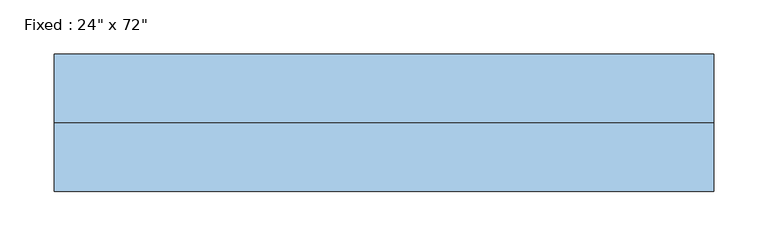
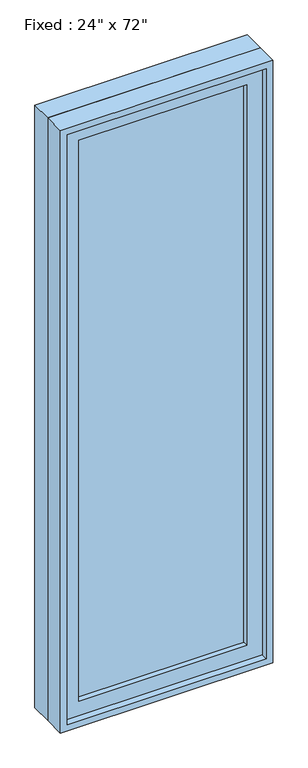
"""IFC4 building model written with IfcOpenShell, lengths in millimetres: window geometry."""

from ifc_helpers import new_model, si_unit, frame, origin, place, context, project, spatial, polyline, outline, extrude, source, transform, mapped, element, save


def window_78893e6c(model_context):
    return source(origin(), model_context, "Body", "SweptSolid", [
        extrude(outline(polyline([(203.2, -15.875), (203.2, -28.575), (-279.4, -28.575), (-279.4, -15.875), (203.2, -15.875)])), frame((0.0, 0.0, 368.3), z_axis=(0.0, 0.0, 1.0), x_axis=(1.0, 0.0, 0.0)), (0.0, 0.0, 1.0), 1701.8),
        extrude(outline(polyline([(2114.55, -323.85), (323.85, -323.85), (323.85, 247.65), (2114.55, 247.65), (2114.55, -323.85)]), holes=[polyline([(2070.1, -279.4), (2070.1, 203.2), (368.3, 203.2), (368.3, -279.4), (2070.1, -279.4)])]), frame((0.0, -44.45, 0.0), z_axis=(0.0, 1.0, 0.0), x_axis=(0.0, 0.0, 1.0)), (0.0, 0.0, 1.0), 44.45),
        extrude(outline(polyline([(2133.6, -342.9), (304.8, -342.9), (304.8, 266.7), (2133.6, 266.7), (2133.6, -342.9)]), holes=[polyline([(2101.85, -311.15), (2101.85, 234.95), (336.55, 234.95), (336.55, -311.15), (2101.85, -311.15)])]), frame((0.0, 0.0, 0.0), z_axis=(0.0, 1.0, 0.0), x_axis=(0.0, 0.0, 1.0)), (0.0, 0.0, 1.0), 63.5),
        extrude(outline(polyline([(2133.6, 266.7), (2133.6, -342.9), (304.8, -342.9), (304.8, 266.7), (2133.6, 266.7)]), holes=[polyline([(2114.55, 247.65), (323.85, 247.65), (323.85, -323.85), (2114.55, -323.85), (2114.55, 247.65)])]), frame((0.0, -63.5, 0.0), z_axis=(0.0, 1.0, 0.0), x_axis=(0.0, 0.0, 1.0)), (0.0, 0.0, 1.0), 63.5),
    ])


if __name__ == "__main__":
    model = new_model("IFC4")
    model_context = context("Model", 3, world=origin())
    ifc_project = project(units=[si_unit("LENGTHUNIT", "METRE", prefix="MILLI")], contexts=[model_context])
    site = spatial("IfcSite", under=ifc_project)
    building = spatial("IfcBuilding", under=site)
    placement = place(None, origin())
    window_shape = window_78893e6c(model_context)
    element("IfcWindow", 1, ObjectType="Fixed : 24\" x 72\"", at=placement, inside=building, context=model_context, shape_type="MappedRepresentation", body=[
        mapped(window_shape, transform((0.0, 0.0, 0.0), x_axis=(1.0, 0.0, 0.0), y_axis=(0.0, 1.0, 0.0), z_axis=(0.0, 0.0, 1.0))),
    ])
    save(model, "model.ifc")

# Revit data of these elements
# Type "Fixed : 24\" x 72\""
#   Type Mark = "7"
#   Construction Type Id = "GSP4R"
#   Assembly Code = "B2020100"
#   Analytic Construction = "1/8 in Pilkington single glazing"
#   Visual Light Transmittance = 0.9
#   Solar Heat Gain Coefficient = 0.78
#   Heat Transfer Coefficient (U) = 0.6496 BTU/(h·ft²·°F)
#   Height = 6' - 0"
#   Default Sill Height = 1' - 0"
#   Width = 2' - 0"
#   Window Inset = 0' - 0 3/4"
#   Define Thermal Properties by = 1
#   Define Thermal Properties by = 1
#   Glass Pane Material = Glass
#   Sash Material = Sash
#   Wall Closure = (empty or 0)
# Element 1 (IfcWindow, "Fixed : 24\" x 72\"")
#   Materials on its faces: "Sash", "Glass"
# Materials
#   "Glass": class "Glass", colour RGB 0 128 192, transparency 0.75, Description = "Soda Lime Glass", Cost = 0
#   "Sash": class "Wood", colour RGB 224 178 126, transparency 0, Cost = 0
